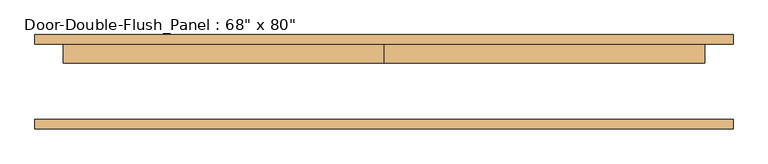
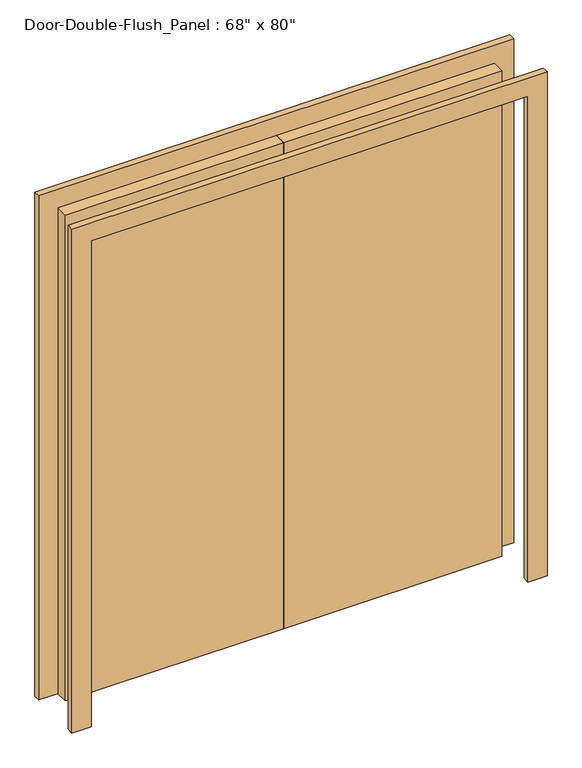
"""IFC4 building model written with IfcOpenShell, lengths in millimetres: door geometry."""

from ifc_helpers import new_model, si_unit, frame, origin, origin_with_axes, place, context, project, spatial, polyline, outline, extrude, source, transform, mapped, element, save


def door_aae36eb6(model_context):
    return source(origin(), model_context, "Body", "SweptSolid", [
        extrude(outline(polyline([(2032.0, -863.6), (2032.0, 863.6), (0.0, 863.6), (0.0, 939.8), (2108.2, 939.8), (2108.2, -939.8), (0.0, -939.8), (0.0, -863.6), (2032.0, -863.6)])), frame((0.0, -127.0, 0.0), z_axis=(0.0, 1.0, 0.0), x_axis=(0.0, 0.0, 1.0)), (0.0, 0.0, 1.0), 25.4),
        extrude(outline(polyline([(2032.0, -863.6), (2032.0, 863.6), (0.0, 863.6), (0.0, 939.8), (2108.2, 939.8), (2108.2, -939.8), (0.0, -939.8), (0.0, -863.6), (2032.0, -863.6)])), frame((0.0, 101.6, 0.0), z_axis=(0.0, 1.0, 0.0), x_axis=(0.0, 0.0, 1.0)), (0.0, 0.0, 1.0), 25.4),
        extrude(outline(polyline([(0.0, 101.6), (863.6, 101.6), (863.6, 50.8), (0.0, 50.8), (0.0, 101.6)])), origin_with_axes(), (0.0, 0.0, 1.0), 2032.0),
        extrude(outline(polyline([(-863.6, 101.6), (0.0, 101.6), (0.0, 50.8), (-863.6, 50.8), (-863.6, 101.6)])), origin_with_axes(), (0.0, 0.0, 1.0), 2032.0),
    ])


if __name__ == "__main__":
    model = new_model("IFC4")
    model_context = context("Model", 3, world=origin())
    ifc_project = project(units=[si_unit("LENGTHUNIT", "METRE", prefix="MILLI")], contexts=[model_context])
    site = spatial("IfcSite", under=ifc_project)
    building = spatial("IfcBuilding", under=site)
    placement = place(None, origin())
    door_shape = door_aae36eb6(model_context)
    element("IfcDoor", 1, ObjectType="Door-Double-Flush_Panel : 68\" x 80\"", at=placement, inside=building, context=model_context, shape_type="MappedRepresentation", body=[
        mapped(door_shape, transform((0.0, 0.0, 0.0), x_axis=(1.0, 0.0, 0.0), y_axis=(0.0, 1.0, 0.0), z_axis=(0.0, 0.0, 1.0))),
    ])
    save(model, "model.ifc")

# Revit data of these elements
# Type "Door-Double-Flush_Panel : 68\" x 80\""
#   Type Mark = "8"
#   Construction Type Id = "DOOR"
#   Assembly Code = "C1020"
#   Analytic Construction = "Wooden"
#   Thickness = 0' - 2"
#   Thermal Resistance (R) = 2.5876 (h·ft²·°F)/BTU
#   Swing Angle [instance default] = 90.00°
#   Panel Width = 2' - 10"
#   Heat Transfer Coefficient (U) = 0.3865 BTU/(h·ft²·°F)
#   Height = 6' - 8"
#   Trim Projection Ext = 0' - 1"
#   Trim Projection Int = 0' - 1"
#   Trim Width = 0' - 3"
#   Width = 5' - 8"
#   Define Thermal Properties by = 1
#   Panel Material = Wood - Birch - Solid Stained Light Low Gloss
#   Trim Material = Paint - Sienna
#   Visual Light Transmittance = 0
#   Solar Heat Gain Coefficient = 0
#   Function = (empty or 0)
#   Wall Closure = (empty or 0)
# Element 1 (IfcDoor, "Door-Double-Flush_Panel : 68\" x 80\"")
#   Materials on its faces: "Paint - Sienna", "Wood - Birch - Solid Stained Light Low Gloss"
# Materials
#   "Wood - Birch - Solid Stained Light Low Gloss": class "Wood", colour RGB 210 159 95, transparency 0, Cost = 0
#   "Paint - Sienna": colour RGB 118 70 51, transparency 0, Cost = 0
